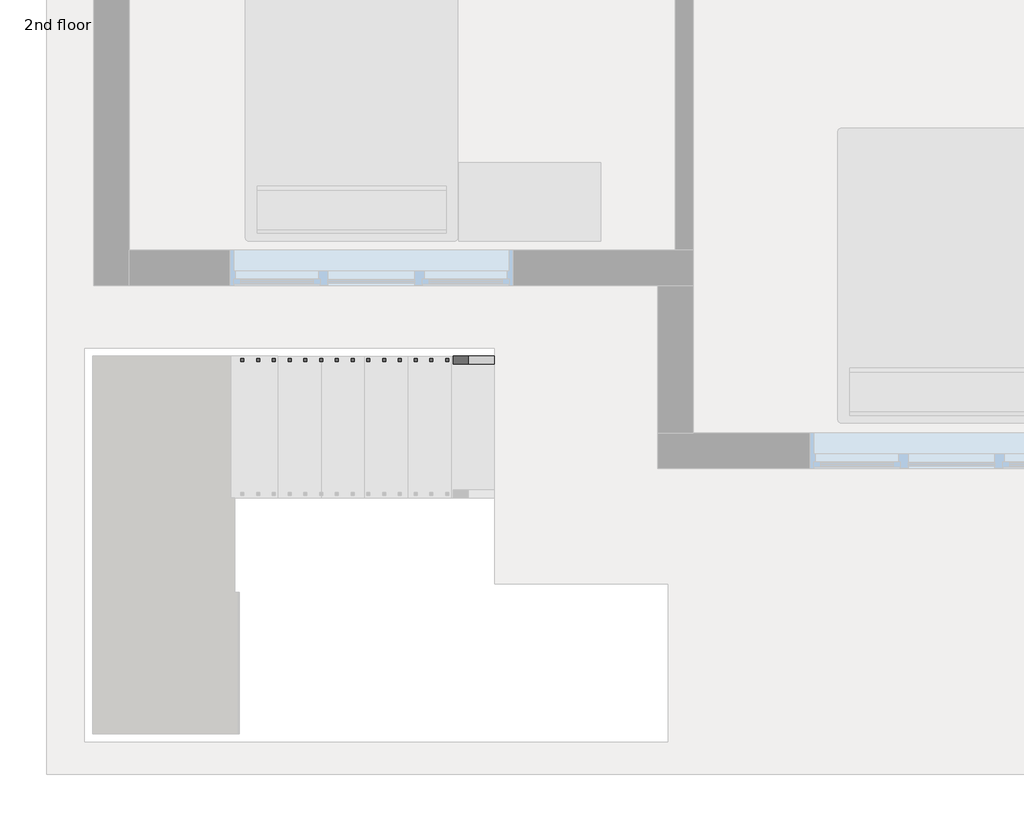
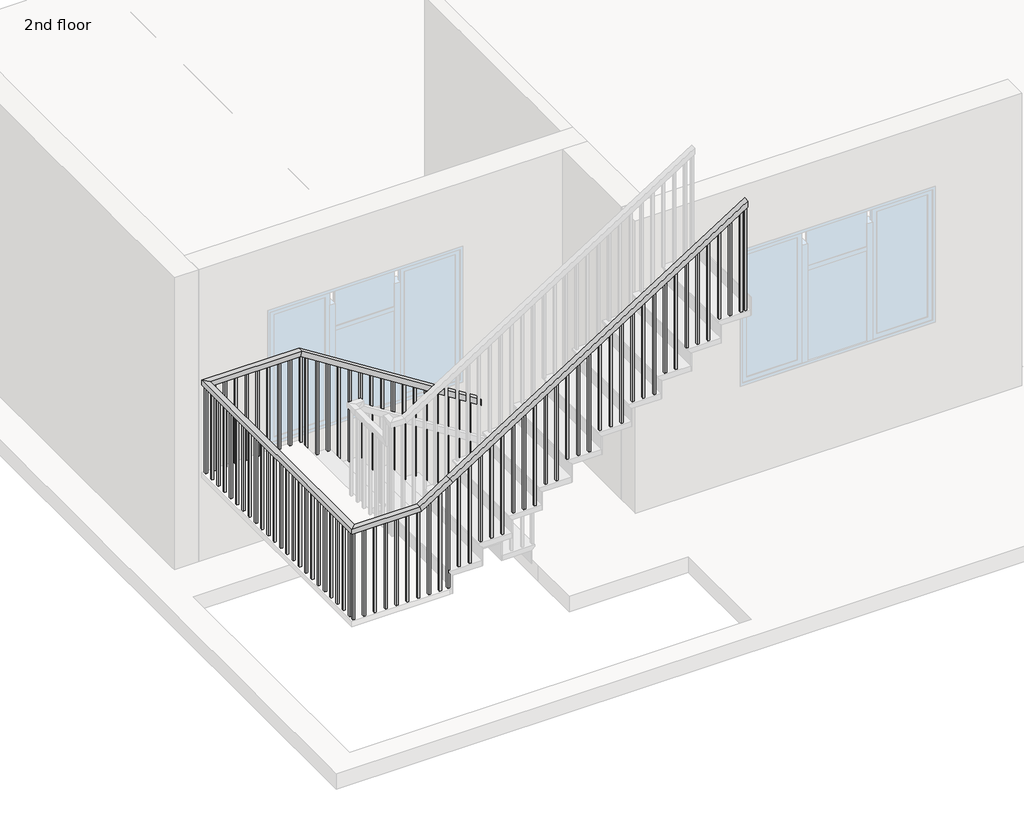
# One storey, part 3 of 4: 1 railing.
"""IFC4 building model written with IfcOpenShell, lengths in millimetres."""

from ifc_helpers import new_model, si_unit, frame, origin, place, context, project, spatial, polyline, outline, extrude, faceted_brep, element, save

model = new_model("IFC4")

# Units and contexts
model_context = context("Model", 3, world=origin())
ifc_project = project(units=[si_unit("LENGTHUNIT", "METRE", prefix="MILLI")], contexts=[model_context])

# Site, building, storey
site = spatial("IfcSite", under=ifc_project)
building = spatial("IfcBuilding", under=site)
storey = spatial("IfcBuildingStorey", under=building, Name="2nd floor", Elevation=7010.4)

# Railing
placement = place(None, origin())
element("IfcRailing", 1, ObjectType="Handrail - Rectangular", at=placement, inside=storey, context=model_context, shape_type="SolidModel", body=[
    faceted_brep([(-6576.0763529, -1102.4338022, 8102.6), (-6576.0763529, -1102.4338022, 8042.386276), (-6576.0763529, -1051.6338022, 8042.386276), (-6576.0763529, -1051.6338022, 8102.6), (-8252.4763529, -1102.4338022, 9169.4), (-8267.2693478, -1102.4338022, 9118.6), (-8267.2693478, -1051.6338022, 9118.6), (-8252.4763529, -1051.6338022, 9169.4), (-9116.0763529, -1102.4338022, 9169.4), (-9116.0763529, -1102.4338022, 9118.6), (-9166.8763529, -1051.6338022, 9118.6), (-9166.8763529, -1051.6338022, 9169.4), (-9116.0763529, -3439.2338022, 9169.4), (-9116.0763529, -3439.2338022, 9118.6), (-9166.8763529, -3490.0338022, 9118.6), (-9166.8763529, -3490.0338022, 9169.4), (-8531.8763529, -3439.2338022, 9169.4), (-8517.083358, -3439.2338022, 9118.6), (-8517.083358, -3490.0338022, 9118.6), (-8531.8763529, -3490.0338022, 9169.4), (-8252.4763529, -3439.2338022, 9347.2), (-8225.2030779, -3439.2338022, 9304.3419964), (-8225.2030779, -3490.0338022, 9304.3419964), (-8252.4763529, -3490.0338022, 9347.2), (-5458.4763529, -3439.2338022, 11125.2), (-5458.4763529, -3490.0338022, 11125.2), (-5458.4763529, -3490.0338022, 11064.986276), (-5458.4763529, -3439.2338022, 11064.986276)], [[[0, 1, 2, 3]], [[1, 0, 4, 5]], [[2, 1, 5, 6]], [[3, 2, 6, 7]], [[0, 3, 7, 4]], [[5, 4, 8, 9]], [[6, 5, 9, 10]], [[7, 6, 10, 11]], [[4, 7, 11, 8]], [[9, 8, 12, 13]], [[10, 9, 13, 14]], [[11, 10, 14, 15]], [[8, 11, 15, 12]], [[13, 12, 16, 17]], [[14, 13, 17, 18]], [[15, 14, 18, 19]], [[12, 15, 19, 16]], [[17, 16, 20, 21]], [[18, 17, 21, 22]], [[19, 18, 22, 23]], [[16, 19, 23, 20]], [[24, 25, 26, 27]], [[21, 20, 24, 27]], [[22, 21, 27, 26]], [[23, 22, 26, 25]], [[20, 23, 25, 24]]]),
    extrude(outline(polyline([(11038.7203669, -5499.7513529), (11026.5976396, -5518.8013529), (10033.0, -5518.8013529), (10033.0, -5499.7513529), (11038.7203669, -5499.7513529)])), frame((0.0, -3474.1588022, 0.0), z_axis=(0.0, 1.0, 0.0), x_axis=(0.0, 0.0, 1.0)), (0.0, 0.0, 1.0), 19.05),
    extrude(outline(polyline([(10974.0658214, -5601.3513529), (10961.9430941, -5620.4013529), (10033.0, -5620.4013529), (10033.0, -5601.3513529), (10974.0658214, -5601.3513529)])), frame((0.0, -3474.1588022, 0.0), z_axis=(0.0, 1.0, 0.0), x_axis=(0.0, 0.0, 1.0)), (0.0, 0.0, 1.0), 19.05),
    extrude(outline(polyline([(10909.411276, -5702.9513529), (10897.2885487, -5722.0013529), (10033.0, -5722.0013529), (10033.0, -5702.9513529), (10909.411276, -5702.9513529)])), frame((0.0, -3474.1588022, 0.0), z_axis=(0.0, 1.0, 0.0), x_axis=(0.0, 0.0, 1.0)), (0.0, 0.0, 1.0), 19.05),
    extrude(outline(polyline([(10844.7567305, -5804.5513529), (10832.6340032, -5823.6013529), (9855.2, -5823.6013529), (9855.2, -5804.5513529), (10844.7567305, -5804.5513529)])), frame((0.0, -3474.1588022, 0.0), z_axis=(0.0, 1.0, 0.0), x_axis=(0.0, 0.0, 1.0)), (0.0, 0.0, 1.0), 19.05),
    extrude(outline(polyline([(10780.1021851, -5906.1513529), (10767.9794578, -5925.2013529), (9855.2, -5925.2013529), (9855.2, -5906.1513529), (10780.1021851, -5906.1513529)])), frame((0.0, -3474.1588022, 0.0), z_axis=(0.0, 1.0, 0.0), x_axis=(0.0, 0.0, 1.0)), (0.0, 0.0, 1.0), 19.05),
    extrude(outline(polyline([(10715.4476396, -6007.7513529), (10703.3249123, -6026.8013529), (9855.2, -6026.8013529), (9855.2, -6007.7513529), (10715.4476396, -6007.7513529)])), frame((0.0, -3474.1588022, 0.0), z_axis=(0.0, 1.0, 0.0), x_axis=(0.0, 0.0, 1.0)), (0.0, 0.0, 1.0), 19.05),
    extrude(outline(polyline([(10650.7930941, -6109.3513529), (10638.6703669, -6128.4013529), (9677.4, -6128.4013529), (9677.4, -6109.3513529), (10650.7930941, -6109.3513529)])), frame((0.0, -3474.1588022, 0.0), z_axis=(0.0, 1.0, 0.0), x_axis=(0.0, 0.0, 1.0)), (0.0, 0.0, 1.0), 19.05),
    extrude(outline(polyline([(10586.1385487, -6210.9513529), (10574.0158214, -6230.0013529), (9677.4, -6230.0013529), (9677.4, -6210.9513529), (10586.1385487, -6210.9513529)])), frame((0.0, -3474.1588022, 0.0), z_axis=(0.0, 1.0, 0.0), x_axis=(0.0, 0.0, 1.0)), (0.0, 0.0, 1.0), 19.05),
    extrude(outline(polyline([(10521.4840032, -6312.5513529), (10509.361276, -6331.6013529), (9499.6, -6331.6013529), (9499.6, -6312.5513529), (10521.4840032, -6312.5513529)])), frame((0.0, -3474.1588022, 0.0), z_axis=(0.0, 1.0, 0.0), x_axis=(0.0, 0.0, 1.0)), (0.0, 0.0, 1.0), 19.05),
    extrude(outline(polyline([(10456.8294578, -6414.1513529), (10444.7067305, -6433.2013529), (9499.6, -6433.2013529), (9499.6, -6414.1513529), (10456.8294578, -6414.1513529)])), frame((0.0, -3474.1588022, 0.0), z_axis=(0.0, 1.0, 0.0), x_axis=(0.0, 0.0, 1.0)), (0.0, 0.0, 1.0), 19.05),
    extrude(outline(polyline([(10392.1749123, -6515.7513529), (10380.0521851, -6534.8013529), (9499.6, -6534.8013529), (9499.6, -6515.7513529), (10392.1749123, -6515.7513529)])), frame((0.0, -3474.1588022, 0.0), z_axis=(0.0, 1.0, 0.0), x_axis=(0.0, 0.0, 1.0)), (0.0, 0.0, 1.0), 19.05),
    extrude(outline(polyline([(10327.5203669, -6617.3513529), (10315.3976396, -6636.4013529), (9321.8, -6636.4013529), (9321.8, -6617.3513529), (10327.5203669, -6617.3513529)])), frame((0.0, -3474.1588022, 0.0), z_axis=(0.0, 1.0, 0.0), x_axis=(0.0, 0.0, 1.0)), (0.0, 0.0, 1.0), 19.05),
    extrude(outline(polyline([(10262.8658214, -6718.9513529), (10250.7430941, -6738.0013529), (9321.8, -6738.0013529), (9321.8, -6718.9513529), (10262.8658214, -6718.9513529)])), frame((0.0, -3474.1588022, 0.0), z_axis=(0.0, 1.0, 0.0), x_axis=(0.0, 0.0, 1.0)), (0.0, 0.0, 1.0), 19.05),
    extrude(outline(polyline([(10198.211276, -6820.5513529), (10186.0885487, -6839.6013529), (9321.8, -6839.6013529), (9321.8, -6820.5513529), (10198.211276, -6820.5513529)])), frame((0.0, -3474.1588022, 0.0), z_axis=(0.0, 1.0, 0.0), x_axis=(0.0, 0.0, 1.0)), (0.0, 0.0, 1.0), 19.05),
    extrude(outline(polyline([(10133.5567305, -6922.1513529), (10121.4340032, -6941.2013529), (9144.0, -6941.2013529), (9144.0, -6922.1513529), (10133.5567305, -6922.1513529)])), frame((0.0, -3474.1588022, 0.0), z_axis=(0.0, 1.0, 0.0), x_axis=(0.0, 0.0, 1.0)), (0.0, 0.0, 1.0), 19.05),
    extrude(outline(polyline([(10068.9021851, -7023.7513529), (10056.7794578, -7042.8013529), (9144.0, -7042.8013529), (9144.0, -7023.7513529), (10068.9021851, -7023.7513529)])), frame((0.0, -3474.1588022, 0.0), z_axis=(0.0, 1.0, 0.0), x_axis=(0.0, 0.0, 1.0)), (0.0, 0.0, 1.0), 19.05),
    extrude(outline(polyline([(10004.2476396, -7125.3513529), (9992.1249123, -7144.4013529), (9144.0, -7144.4013529), (9144.0, -7125.3513529), (10004.2476396, -7125.3513529)])), frame((0.0, -3474.1588022, 0.0), z_axis=(0.0, 1.0, 0.0), x_axis=(0.0, 0.0, 1.0)), (0.0, 0.0, 1.0), 19.05),
    extrude(outline(polyline([(9939.5930941, -7226.9513529), (9927.4703669, -7246.0013529), (8966.2, -7246.0013529), (8966.2, -7226.9513529), (9939.5930941, -7226.9513529)])), frame((0.0, -3474.1588022, 0.0), z_axis=(0.0, 1.0, 0.0), x_axis=(0.0, 0.0, 1.0)), (0.0, 0.0, 1.0), 19.05),
    extrude(outline(polyline([(9874.9385487, -7328.5513529), (9862.8158214, -7347.6013529), (8966.2, -7347.6013529), (8966.2, -7328.5513529), (9874.9385487, -7328.5513529)])), frame((0.0, -3474.1588022, 0.0), z_axis=(0.0, 1.0, 0.0), x_axis=(0.0, 0.0, 1.0)), (0.0, 0.0, 1.0), 19.05),
    extrude(outline(polyline([(9810.2840032, -7430.1513529), (9798.161276, -7449.2013529), (8788.4, -7449.2013529), (8788.4, -7430.1513529), (9810.2840032, -7430.1513529)])), frame((0.0, -3474.1588022, 0.0), z_axis=(0.0, 1.0, 0.0), x_axis=(0.0, 0.0, 1.0)), (0.0, 0.0, 1.0), 19.05),
    extrude(outline(polyline([(9745.6294578, -7531.7513529), (9733.5067305, -7550.8013529), (8788.4, -7550.8013529), (8788.4, -7531.7513529), (9745.6294578, -7531.7513529)])), frame((0.0, -3474.1588022, 0.0), z_axis=(0.0, 1.0, 0.0), x_axis=(0.0, 0.0, 1.0)), (0.0, 0.0, 1.0), 19.05),
    extrude(outline(polyline([(9680.9749123, -7633.3513529), (9668.8521851, -7652.4013529), (8788.4, -7652.4013529), (8788.4, -7633.3513529), (9680.9749123, -7633.3513529)])), frame((0.0, -3474.1588022, 0.0), z_axis=(0.0, 1.0, 0.0), x_axis=(0.0, 0.0, 1.0)), (0.0, 0.0, 1.0), 19.05),
    extrude(outline(polyline([(9616.3203669, -7734.9513529), (9604.1976396, -7754.0013529), (8610.6, -7754.0013529), (8610.6, -7734.9513529), (9616.3203669, -7734.9513529)])), frame((0.0, -3474.1588022, 0.0), z_axis=(0.0, 1.0, 0.0), x_axis=(0.0, 0.0, 1.0)), (0.0, 0.0, 1.0), 19.05),
    extrude(outline(polyline([(9551.6658214, -7836.5513529), (9539.5430941, -7855.6013529), (8610.6, -7855.6013529), (8610.6, -7836.5513529), (9551.6658214, -7836.5513529)])), frame((0.0, -3474.1588022, 0.0), z_axis=(0.0, 1.0, 0.0), x_axis=(0.0, 0.0, 1.0)), (0.0, 0.0, 1.0), 19.05),
    extrude(outline(polyline([(9487.011276, -7938.1513529), (9474.8885487, -7957.2013529), (8610.6, -7957.2013529), (8610.6, -7938.1513529), (9487.011276, -7938.1513529)])), frame((0.0, -3474.1588022, 0.0), z_axis=(0.0, 1.0, 0.0), x_axis=(0.0, 0.0, 1.0)), (0.0, 0.0, 1.0), 19.05),
    extrude(outline(polyline([(9422.3567305, -8039.7513529), (9410.2340032, -8058.8013529), (8432.8, -8058.8013529), (8432.8, -8039.7513529), (9422.3567305, -8039.7513529)])), frame((0.0, -3474.1588022, 0.0), z_axis=(0.0, 1.0, 0.0), x_axis=(0.0, 0.0, 1.0)), (0.0, 0.0, 1.0), 19.05),
    extrude(outline(polyline([(9357.7021851, -8141.3513529), (9345.5794578, -8160.4013529), (8432.8, -8160.4013529), (8432.8, -8141.3513529), (9357.7021851, -8141.3513529)])), frame((0.0, -3474.1588022, 0.0), z_axis=(0.0, 1.0, 0.0), x_axis=(0.0, 0.0, 1.0)), (0.0, 0.0, 1.0), 19.05),
    extrude(outline(polyline([(9244.5567305, -8319.1513529), (9232.4340032, -8338.2013529), (8255.0, -8338.2013529), (8255.0, -8319.1513529), (9244.5567305, -8319.1513529)])), frame((0.0, -3474.1588022, 0.0), z_axis=(0.0, 1.0, 0.0), x_axis=(0.0, 0.0, 1.0)), (0.0, 0.0, 1.0), 19.05),
    extrude(outline(polyline([(9179.9021851, -8420.7513529), (9167.7794578, -8439.8013529), (8255.0, -8439.8013529), (8255.0, -8420.7513529), (9179.9021851, -8420.7513529)])), frame((0.0, -3474.1588022, 0.0), z_axis=(0.0, 1.0, 0.0), x_axis=(0.0, 0.0, 1.0)), (0.0, 0.0, 1.0), 19.05),
    extrude(outline(polyline([(-8541.4013529, -3474.1588022), (-8541.4013529, -3455.1088022), (-8522.3513529, -3455.1088022), (-8522.3513529, -3474.1588022), (-8541.4013529, -3474.1588022)])), frame((0.0, 0.0, 8255.0), z_axis=(0.0, 0.0, 1.0), x_axis=(1.0, 0.0, 0.0)), (0.0, 0.0, 1.0), 863.6),
    extrude(outline(polyline([(-8643.0013529, -3474.1588022), (-8643.0013529, -3455.1088022), (-8623.9513529, -3455.1088022), (-8623.9513529, -3474.1588022), (-8643.0013529, -3474.1588022)])), frame((0.0, 0.0, 8255.0), z_axis=(0.0, 0.0, 1.0), x_axis=(1.0, 0.0, 0.0)), (0.0, 0.0, 1.0), 863.6),
    extrude(outline(polyline([(-8744.6013529, -3474.1588022), (-8744.6013529, -3455.1088022), (-8725.5513529, -3455.1088022), (-8725.5513529, -3474.1588022), (-8744.6013529, -3474.1588022)])), frame((0.0, 0.0, 8255.0), z_axis=(0.0, 0.0, 1.0), x_axis=(1.0, 0.0, 0.0)), (0.0, 0.0, 1.0), 863.6),
    extrude(outline(polyline([(-8846.2013529, -3474.1588022), (-8846.2013529, -3455.1088022), (-8827.1513529, -3455.1088022), (-8827.1513529, -3474.1588022), (-8846.2013529, -3474.1588022)])), frame((0.0, 0.0, 8255.0), z_axis=(0.0, 0.0, 1.0), x_axis=(1.0, 0.0, 0.0)), (0.0, 0.0, 1.0), 863.6),
    extrude(outline(polyline([(-8947.8013529, -3474.1588022), (-8947.8013529, -3455.1088022), (-8928.7513529, -3455.1088022), (-8928.7513529, -3474.1588022), (-8947.8013529, -3474.1588022)])), frame((0.0, 0.0, 8255.0), z_axis=(0.0, 0.0, 1.0), x_axis=(1.0, 0.0, 0.0)), (0.0, 0.0, 1.0), 863.6),
    extrude(outline(polyline([(-9049.4013529, -3474.1588022), (-9049.4013529, -3455.1088022), (-9030.3513529, -3455.1088022), (-9030.3513529, -3474.1588022), (-9049.4013529, -3474.1588022)])), frame((0.0, 0.0, 8255.0), z_axis=(0.0, 0.0, 1.0), x_axis=(1.0, 0.0, 0.0)), (0.0, 0.0, 1.0), 863.6),
    extrude(outline(polyline([(-9151.0013529, -3404.3088022), (-9131.9513529, -3404.3088022), (-9131.9513529, -3423.3588022), (-9151.0013529, -3423.3588022), (-9151.0013529, -3404.3088022)])), frame((0.0, 0.0, 8255.0), z_axis=(0.0, 0.0, 1.0), x_axis=(1.0, 0.0, 0.0)), (0.0, 0.0, 1.0), 863.6),
    extrude(outline(polyline([(-9151.0013529, -3302.7088022), (-9131.9513529, -3302.7088022), (-9131.9513529, -3321.7588022), (-9151.0013529, -3321.7588022), (-9151.0013529, -3302.7088022)])), frame((0.0, 0.0, 8255.0), z_axis=(0.0, 0.0, 1.0), x_axis=(1.0, 0.0, 0.0)), (0.0, 0.0, 1.0), 863.6),
    extrude(outline(polyline([(-9151.0013529, -3201.1088022), (-9131.9513529, -3201.1088022), (-9131.9513529, -3220.1588022), (-9151.0013529, -3220.1588022), (-9151.0013529, -3201.1088022)])), frame((0.0, 0.0, 8255.0), z_axis=(0.0, 0.0, 1.0), x_axis=(1.0, 0.0, 0.0)), (0.0, 0.0, 1.0), 863.6),
    extrude(outline(polyline([(-9151.0013529, -3099.5088022), (-9131.9513529, -3099.5088022), (-9131.9513529, -3118.5588022), (-9151.0013529, -3118.5588022), (-9151.0013529, -3099.5088022)])), frame((0.0, 0.0, 8255.0), z_axis=(0.0, 0.0, 1.0), x_axis=(1.0, 0.0, 0.0)), (0.0, 0.0, 1.0), 863.6),
    extrude(outline(polyline([(-9151.0013529, -2997.9088022), (-9131.9513529, -2997.9088022), (-9131.9513529, -3016.9588022), (-9151.0013529, -3016.9588022), (-9151.0013529, -2997.9088022)])), frame((0.0, 0.0, 8255.0), z_axis=(0.0, 0.0, 1.0), x_axis=(1.0, 0.0, 0.0)), (0.0, 0.0, 1.0), 863.6),
    extrude(outline(polyline([(-9151.0013529, -2896.3088022), (-9131.9513529, -2896.3088022), (-9131.9513529, -2915.3588022), (-9151.0013529, -2915.3588022), (-9151.0013529, -2896.3088022)])), frame((0.0, 0.0, 8255.0), z_axis=(0.0, 0.0, 1.0), x_axis=(1.0, 0.0, 0.0)), (0.0, 0.0, 1.0), 863.6),
    extrude(outline(polyline([(-9151.0013529, -2794.7088022), (-9131.9513529, -2794.7088022), (-9131.9513529, -2813.7588022), (-9151.0013529, -2813.7588022), (-9151.0013529, -2794.7088022)])), frame((0.0, 0.0, 8255.0), z_axis=(0.0, 0.0, 1.0), x_axis=(1.0, 0.0, 0.0)), (0.0, 0.0, 1.0), 863.6),
    extrude(outline(polyline([(-9151.0013529, -2693.1088022), (-9131.9513529, -2693.1088022), (-9131.9513529, -2712.1588022), (-9151.0013529, -2712.1588022), (-9151.0013529, -2693.1088022)])), frame((0.0, 0.0, 8255.0), z_axis=(0.0, 0.0, 1.0), x_axis=(1.0, 0.0, 0.0)), (0.0, 0.0, 1.0), 863.6),
    extrude(outline(polyline([(-9151.0013529, -2591.5088022), (-9131.9513529, -2591.5088022), (-9131.9513529, -2610.5588022), (-9151.0013529, -2610.5588022), (-9151.0013529, -2591.5088022)])), frame((0.0, 0.0, 8255.0), z_axis=(0.0, 0.0, 1.0), x_axis=(1.0, 0.0, 0.0)), (0.0, 0.0, 1.0), 863.6),
    extrude(outline(polyline([(-9151.0013529, -2489.9088022), (-9131.9513529, -2489.9088022), (-9131.9513529, -2508.9588022), (-9151.0013529, -2508.9588022), (-9151.0013529, -2489.9088022)])), frame((0.0, 0.0, 8255.0), z_axis=(0.0, 0.0, 1.0), x_axis=(1.0, 0.0, 0.0)), (0.0, 0.0, 1.0), 863.6),
    extrude(outline(polyline([(-9151.0013529, -2388.3088022), (-9131.9513529, -2388.3088022), (-9131.9513529, -2407.3588022), (-9151.0013529, -2407.3588022), (-9151.0013529, -2388.3088022)])), frame((0.0, 0.0, 8255.0), z_axis=(0.0, 0.0, 1.0), x_axis=(1.0, 0.0, 0.0)), (0.0, 0.0, 1.0), 863.6),
    extrude(outline(polyline([(-9151.0013529, -2286.7088022), (-9131.9513529, -2286.7088022), (-9131.9513529, -2305.7588022), (-9151.0013529, -2305.7588022), (-9151.0013529, -2286.7088022)])), frame((0.0, 0.0, 8255.0), z_axis=(0.0, 0.0, 1.0), x_axis=(1.0, 0.0, 0.0)), (0.0, 0.0, 1.0), 863.6),
    extrude(outline(polyline([(-9151.0013529, -2185.1088022), (-9131.9513529, -2185.1088022), (-9131.9513529, -2204.1588022), (-9151.0013529, -2204.1588022), (-9151.0013529, -2185.1088022)])), frame((0.0, 0.0, 8255.0), z_axis=(0.0, 0.0, 1.0), x_axis=(1.0, 0.0, 0.0)), (0.0, 0.0, 1.0), 863.6),
    extrude(outline(polyline([(-9151.0013529, -2083.5088022), (-9131.9513529, -2083.5088022), (-9131.9513529, -2102.5588022), (-9151.0013529, -2102.5588022), (-9151.0013529, -2083.5088022)])), frame((0.0, 0.0, 8255.0), z_axis=(0.0, 0.0, 1.0), x_axis=(1.0, 0.0, 0.0)), (0.0, 0.0, 1.0), 863.6),
    extrude(outline(polyline([(-9151.0013529, -1981.9088022), (-9131.9513529, -1981.9088022), (-9131.9513529, -2000.9588022), (-9151.0013529, -2000.9588022), (-9151.0013529, -1981.9088022)])), frame((0.0, 0.0, 8255.0), z_axis=(0.0, 0.0, 1.0), x_axis=(1.0, 0.0, 0.0)), (0.0, 0.0, 1.0), 863.6),
    extrude(outline(polyline([(-9151.0013529, -1880.3088022), (-9131.9513529, -1880.3088022), (-9131.9513529, -1899.3588022), (-9151.0013529, -1899.3588022), (-9151.0013529, -1880.3088022)])), frame((0.0, 0.0, 8255.0), z_axis=(0.0, 0.0, 1.0), x_axis=(1.0, 0.0, 0.0)), (0.0, 0.0, 1.0), 863.6),
    extrude(outline(polyline([(-9151.0013529, -1778.7088022), (-9131.9513529, -1778.7088022), (-9131.9513529, -1797.7588022), (-9151.0013529, -1797.7588022), (-9151.0013529, -1778.7088022)])), frame((0.0, 0.0, 8255.0), z_axis=(0.0, 0.0, 1.0), x_axis=(1.0, 0.0, 0.0)), (0.0, 0.0, 1.0), 863.6),
    extrude(outline(polyline([(-9151.0013529, -1677.1088022), (-9131.9513529, -1677.1088022), (-9131.9513529, -1696.1588022), (-9151.0013529, -1696.1588022), (-9151.0013529, -1677.1088022)])), frame((0.0, 0.0, 8255.0), z_axis=(0.0, 0.0, 1.0), x_axis=(1.0, 0.0, 0.0)), (0.0, 0.0, 1.0), 863.6),
    extrude(outline(polyline([(-9151.0013529, -1575.5088022), (-9131.9513529, -1575.5088022), (-9131.9513529, -1594.5588022), (-9151.0013529, -1594.5588022), (-9151.0013529, -1575.5088022)])), frame((0.0, 0.0, 8255.0), z_axis=(0.0, 0.0, 1.0), x_axis=(1.0, 0.0, 0.0)), (0.0, 0.0, 1.0), 863.6),
    extrude(outline(polyline([(-9151.0013529, -1473.9088022), (-9131.9513529, -1473.9088022), (-9131.9513529, -1492.9588022), (-9151.0013529, -1492.9588022), (-9151.0013529, -1473.9088022)])), frame((0.0, 0.0, 8255.0), z_axis=(0.0, 0.0, 1.0), x_axis=(1.0, 0.0, 0.0)), (0.0, 0.0, 1.0), 863.6),
    extrude(outline(polyline([(-9151.0013529, -1372.3088022), (-9131.9513529, -1372.3088022), (-9131.9513529, -1391.3588022), (-9151.0013529, -1391.3588022), (-9151.0013529, -1372.3088022)])), frame((0.0, 0.0, 8255.0), z_axis=(0.0, 0.0, 1.0), x_axis=(1.0, 0.0, 0.0)), (0.0, 0.0, 1.0), 863.6),
    extrude(outline(polyline([(-9151.0013529, -1270.7088022), (-9131.9513529, -1270.7088022), (-9131.9513529, -1289.7588022), (-9151.0013529, -1289.7588022), (-9151.0013529, -1270.7088022)])), frame((0.0, 0.0, 8255.0), z_axis=(0.0, 0.0, 1.0), x_axis=(1.0, 0.0, 0.0)), (0.0, 0.0, 1.0), 863.6),
    extrude(outline(polyline([(-9151.0013529, -1169.1088022), (-9131.9513529, -1169.1088022), (-9131.9513529, -1188.1588022), (-9151.0013529, -1188.1588022), (-9151.0013529, -1169.1088022)])), frame((0.0, 0.0, 8255.0), z_axis=(0.0, 0.0, 1.0), x_axis=(1.0, 0.0, 0.0)), (0.0, 0.0, 1.0), 863.6),
    extrude(outline(polyline([(-9055.7513529, -1067.5088022), (-9055.7513529, -1086.5588022), (-9074.8013529, -1086.5588022), (-9074.8013529, -1067.5088022), (-9055.7513529, -1067.5088022)])), frame((0.0, 0.0, 8255.0), z_axis=(0.0, 0.0, 1.0), x_axis=(1.0, 0.0, 0.0)), (0.0, 0.0, 1.0), 863.6),
    extrude(outline(polyline([(-8954.1513529, -1067.5088022), (-8954.1513529, -1086.5588022), (-8973.2013529, -1086.5588022), (-8973.2013529, -1067.5088022), (-8954.1513529, -1067.5088022)])), frame((0.0, 0.0, 8255.0), z_axis=(0.0, 0.0, 1.0), x_axis=(1.0, 0.0, 0.0)), (0.0, 0.0, 1.0), 863.6),
    extrude(outline(polyline([(-8852.5513529, -1067.5088022), (-8852.5513529, -1086.5588022), (-8871.6013529, -1086.5588022), (-8871.6013529, -1067.5088022), (-8852.5513529, -1067.5088022)])), frame((0.0, 0.0, 8255.0), z_axis=(0.0, 0.0, 1.0), x_axis=(1.0, 0.0, 0.0)), (0.0, 0.0, 1.0), 863.6),
    extrude(outline(polyline([(-8750.9513529, -1067.5088022), (-8750.9513529, -1086.5588022), (-8770.0013529, -1086.5588022), (-8770.0013529, -1067.5088022), (-8750.9513529, -1067.5088022)])), frame((0.0, 0.0, 8255.0), z_axis=(0.0, 0.0, 1.0), x_axis=(1.0, 0.0, 0.0)), (0.0, 0.0, 1.0), 863.6),
    extrude(outline(polyline([(-8649.3513529, -1067.5088022), (-8649.3513529, -1086.5588022), (-8668.4013529, -1086.5588022), (-8668.4013529, -1067.5088022), (-8649.3513529, -1067.5088022)])), frame((0.0, 0.0, 8255.0), z_axis=(0.0, 0.0, 1.0), x_axis=(1.0, 0.0, 0.0)), (0.0, 0.0, 1.0), 863.6),
    extrude(outline(polyline([(-8547.7513529, -1067.5088022), (-8547.7513529, -1086.5588022), (-8566.8013529, -1086.5588022), (-8566.8013529, -1067.5088022), (-8547.7513529, -1067.5088022)])), frame((0.0, 0.0, 8255.0), z_axis=(0.0, 0.0, 1.0), x_axis=(1.0, 0.0, 0.0)), (0.0, 0.0, 1.0), 863.6),
    extrude(outline(polyline([(-8446.1513529, -1067.5088022), (-8446.1513529, -1086.5588022), (-8465.2013529, -1086.5588022), (-8465.2013529, -1067.5088022), (-8446.1513529, -1067.5088022)])), frame((0.0, 0.0, 8255.0), z_axis=(0.0, 0.0, 1.0), x_axis=(1.0, 0.0, 0.0)), (0.0, 0.0, 1.0), 863.6),
    extrude(outline(polyline([(-8344.5513529, -1067.5088022), (-8344.5513529, -1086.5588022), (-8363.6013529, -1086.5588022), (-8363.6013529, -1067.5088022), (-8344.5513529, -1067.5088022)])), frame((0.0, 0.0, 8255.0), z_axis=(0.0, 0.0, 1.0), x_axis=(1.0, 0.0, 0.0)), (0.0, 0.0, 1.0), 863.6),
    extrude(outline(polyline([(9070.7976396, -8192.1513529), (9082.9203669, -8211.2013529), (8077.2, -8211.2013529), (8077.2, -8192.1513529), (9070.7976396, -8192.1513529)])), frame((0.0, -1086.5588022, 0.0), z_axis=(0.0, 1.0, 0.0), x_axis=(0.0, 0.0, 1.0)), (0.0, 0.0, 1.0), 19.05),
    extrude(outline(polyline([(9006.1430941, -8090.5513529), (9018.2658214, -8109.6013529), (8077.2, -8109.6013529), (8077.2, -8090.5513529), (9006.1430941, -8090.5513529)])), frame((0.0, -1086.5588022, 0.0), z_axis=(0.0, 1.0, 0.0), x_axis=(0.0, 0.0, 1.0)), (0.0, 0.0, 1.0), 19.05),
    extrude(outline(polyline([(8941.4885487, -7988.9513529), (8953.611276, -8008.0013529), (8077.2, -8008.0013529), (8077.2, -7988.9513529), (8941.4885487, -7988.9513529)])), frame((0.0, -1086.5588022, 0.0), z_axis=(0.0, 1.0, 0.0), x_axis=(0.0, 0.0, 1.0)), (0.0, 0.0, 1.0), 19.05),
    extrude(outline(polyline([(8876.8340032, -7887.3513529), (8888.9567305, -7906.4013529), (7899.4, -7906.4013529), (7899.4, -7887.3513529), (8876.8340032, -7887.3513529)])), frame((0.0, -1086.5588022, 0.0), z_axis=(0.0, 1.0, 0.0), x_axis=(0.0, 0.0, 1.0)), (0.0, 0.0, 1.0), 19.05),
    extrude(outline(polyline([(8812.1794578, -7785.7513529), (8824.3021851, -7804.8013529), (7899.4, -7804.8013529), (7899.4, -7785.7513529), (8812.1794578, -7785.7513529)])), frame((0.0, -1086.5588022, 0.0), z_axis=(0.0, 1.0, 0.0), x_axis=(0.0, 0.0, 1.0)), (0.0, 0.0, 1.0), 19.05),
    extrude(outline(polyline([(8747.5249123, -7684.1513529), (8759.6476396, -7703.2013529), (7899.4, -7703.2013529), (7899.4, -7684.1513529), (8747.5249123, -7684.1513529)])), frame((0.0, -1086.5588022, 0.0), z_axis=(0.0, 1.0, 0.0), x_axis=(0.0, 0.0, 1.0)), (0.0, 0.0, 1.0), 19.05),
    extrude(outline(polyline([(8682.8703669, -7582.5513529), (8694.9930941, -7601.6013529), (7721.6, -7601.6013529), (7721.6, -7582.5513529), (8682.8703669, -7582.5513529)])), frame((0.0, -1086.5588022, 0.0), z_axis=(0.0, 1.0, 0.0), x_axis=(0.0, 0.0, 1.0)), (0.0, 0.0, 1.0), 19.05),
    extrude(outline(polyline([(8618.2158214, -7480.9513529), (8630.3385487, -7500.0013529), (7721.6, -7500.0013529), (7721.6, -7480.9513529), (8618.2158214, -7480.9513529)])), frame((0.0, -1086.5588022, 0.0), z_axis=(0.0, 1.0, 0.0), x_axis=(0.0, 0.0, 1.0)), (0.0, 0.0, 1.0), 19.05),
    extrude(outline(polyline([(8553.561276, -7379.3513529), (8565.6840032, -7398.4013529), (7543.8, -7398.4013529), (7543.8, -7379.3513529), (8553.561276, -7379.3513529)])), frame((0.0, -1086.5588022, 0.0), z_axis=(0.0, 1.0, 0.0), x_axis=(0.0, 0.0, 1.0)), (0.0, 0.0, 1.0), 19.05),
    extrude(outline(polyline([(8488.9067305, -7277.7513529), (8501.0294578, -7296.8013529), (7543.8, -7296.8013529), (7543.8, -7277.7513529), (8488.9067305, -7277.7513529)])), frame((0.0, -1086.5588022, 0.0), z_axis=(0.0, 1.0, 0.0), x_axis=(0.0, 0.0, 1.0)), (0.0, 0.0, 1.0), 19.05),
    extrude(outline(polyline([(8424.2521851, -7176.1513529), (8436.3749123, -7195.2013529), (7543.8, -7195.2013529), (7543.8, -7176.1513529), (8424.2521851, -7176.1513529)])), frame((0.0, -1086.5588022, 0.0), z_axis=(0.0, 1.0, 0.0), x_axis=(0.0, 0.0, 1.0)), (0.0, 0.0, 1.0), 19.05),
    extrude(outline(polyline([(8359.5976396, -7074.5513529), (8371.7203669, -7093.6013529), (7366.0, -7093.6013529), (7366.0, -7074.5513529), (8359.5976396, -7074.5513529)])), frame((0.0, -1086.5588022, 0.0), z_axis=(0.0, 1.0, 0.0), x_axis=(0.0, 0.0, 1.0)), (0.0, 0.0, 1.0), 19.05),
    extrude(outline(polyline([(8294.9430941, -6972.9513529), (8307.0658214, -6992.0013529), (7366.0, -6992.0013529), (7366.0, -6972.9513529), (8294.9430941, -6972.9513529)])), frame((0.0, -1086.5588022, 0.0), z_axis=(0.0, 1.0, 0.0), x_axis=(0.0, 0.0, 1.0)), (0.0, 0.0, 1.0), 19.05),
    extrude(outline(polyline([(8230.2885487, -6871.3513529), (8242.411276, -6890.4013529), (7366.0, -6890.4013529), (7366.0, -6871.3513529), (8230.2885487, -6871.3513529)])), frame((0.0, -1086.5588022, 0.0), z_axis=(0.0, 1.0, 0.0), x_axis=(0.0, 0.0, 1.0)), (0.0, 0.0, 1.0), 19.05),
    extrude(outline(polyline([(8165.6340032, -6769.7513529), (8177.7567305, -6788.8013529), (7188.2, -6788.8013529), (7188.2, -6769.7513529), (8165.6340032, -6769.7513529)])), frame((0.0, -1086.5588022, 0.0), z_axis=(0.0, 1.0, 0.0), x_axis=(0.0, 0.0, 1.0)), (0.0, 0.0, 1.0), 19.05),
    extrude(outline(polyline([(8100.9794578, -6668.1513529), (8113.1021851, -6687.2013529), (7188.2, -6687.2013529), (7188.2, -6668.1513529), (8100.9794578, -6668.1513529)])), frame((0.0, -1086.5588022, 0.0), z_axis=(0.0, 1.0, 0.0), x_axis=(0.0, 0.0, 1.0)), (0.0, 0.0, 1.0), 19.05),
    extrude(outline(polyline([(9293.0476396, -8242.9513529), (9280.9249123, -8262.0013529), (8255.0, -8262.0013529), (8255.0, -8242.9513529), (9293.0476396, -8242.9513529)])), frame((0.0, -3474.1588022, 0.0), z_axis=(0.0, 1.0, 0.0), x_axis=(0.0, 0.0, 1.0)), (0.0, 0.0, 1.0), 19.05),
    extrude(outline(polyline([(-9151.0013529, -3455.1088022), (-9131.9513529, -3455.1088022), (-9131.9513529, -3474.1588022), (-9151.0013529, -3474.1588022), (-9151.0013529, -3455.1088022)])), frame((0.0, 0.0, 8255.0), z_axis=(0.0, 0.0, 1.0), x_axis=(1.0, 0.0, 0.0)), (0.0, 0.0, 1.0), 863.6),
    extrude(outline(polyline([(-9131.9513529, -1067.5088022), (-9131.9513529, -1086.5588022), (-9151.0013529, -1086.5588022), (-9151.0013529, -1067.5088022), (-9131.9513529, -1067.5088022)])), frame((0.0, 0.0, 8255.0), z_axis=(0.0, 0.0, 1.0), x_axis=(1.0, 0.0, 0.0)), (0.0, 0.0, 1.0), 863.6),
    extrude(outline(polyline([(9103.1249123, -8242.9513529), (9115.2476396, -8262.0013529), (8255.0, -8262.0013529), (8255.0, -8242.9513529), (9103.1249123, -8242.9513529)])), frame((0.0, -1086.5588022, 0.0), z_axis=(0.0, 1.0, 0.0), x_axis=(0.0, 0.0, 1.0)), (0.0, 0.0, 1.0), 19.05),
    extrude(outline(polyline([(11064.986276, -5458.4763529), (11052.8635487, -5477.5263529), (10033.0, -5477.5263529), (10033.0, -5458.4763529), (11064.986276, -5458.4763529)])), frame((0.0, -3474.1588022, 0.0), z_axis=(0.0, 1.0, 0.0), x_axis=(0.0, 0.0, 1.0)), (0.0, 0.0, 1.0), 19.05),
    extrude(outline(polyline([(8042.386276, -6576.0763529), (8054.5090032, -6595.1263529), (7188.2, -6595.1263529), (7188.2, -6576.0763529), (8042.386276, -6576.0763529)])), frame((0.0, -1086.5588022, 0.0), z_axis=(0.0, 1.0, 0.0), x_axis=(0.0, 0.0, 1.0)), (0.0, 0.0, 1.0), 19.05),
])

save(model, "model.ifc")

# Revit data of these elements
# Type "Handrail - Rectangular"
#   Assembly Code = "C2010400"
#   built-in parameter 1008612 = 0.0416667 (stored number, unit not read)
#   built-in parameter 1008611 = 0.0416667 (stored number, unit not read)
#   built-in parameter 1008609 = 0.333333 (stored number, unit not read)
#   built-in parameter 1008604 = 0.166667 (stored number, unit not read)
#   built-in parameter 1008603 = 0.166667 (stored number, unit not read)
#   Railing Height = 3' - 0"
#   built-in parameter 1008630 = 2
#   built-in parameter 1008610 = 2
#   built-in parameter 1008618 = Baluster - Square : 3/4"
# Element 1 (IfcRailing, "Handrail - Rectangular")
#   Phase Created = New Construction
